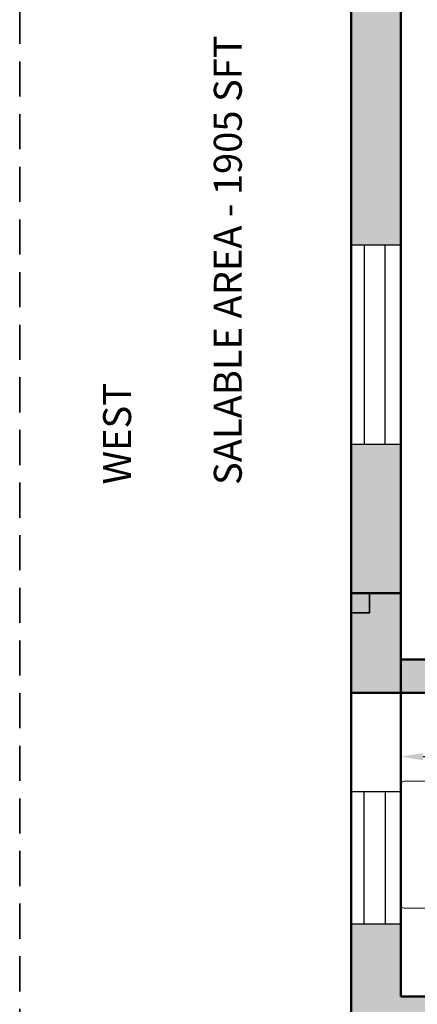
# Model space of a CAD drawing. Units: inches. Extents: x -7 to 1228, y -146 to 1091.
# Tile 50 of 88: x 0 to 72, y 786 to 964. Entities that reach past the tile are written whole.
import ezdxf

# ---------------------------------------------------------------- set-up
doc = ezdxf.new("R2010")
doc.units = ezdxf.units.IN
doc.linetypes.add('DASHED2', pattern=[9.525, 6.35, -3.175])
for name, color, linetype, lineweight in [('A-ANNO-DIMS', 2, 'Continuous', 18), ('A-ANNO-TEXT', 7, 'Continuous', 18), ('A-COLS', 6, 'Continuous', 35), ('A-FLOR-FIXT', 8, 'Continuous', 18), ('A-GLAZ', 175, 'Continuous', 25), ('A-WALL', 7, 'Continuous', 50), ('A-WALL-PATT', 251, 'Continuous', 13), ('C-PROP', 1, 'DASHED2', 35)]:
    doc.layers.add(name, color=color, linetype=linetype, lineweight=lineweight)
doc.styles.get("Standard").update_dxf_attribs({"font": 'arial.ttf'})
doc.dimstyles.new('ISO-25', dxfattribs={"dimtxt": 7, "dimasz": 4, "dimexe": 1.25, "dimexo": 0.625, "dimtad": 1, "dimdec": 1, "dimlunit": 3, "dimtxsty": 'Standard', "dimcen": 2.5, "dimadec": 0, "dimazin": 0, "dimtfac": 1, "dimtdec": 1, "dimtmove": 1, "dimatfit": 3, "dimfxl": 1, "dimarcsym": 0})

# ---------------------------------------------------------------- blocks, each defined once
blk = doc.blocks.new('A$C7B5C7CD4')
at = {"ltscale": 20}
for p, q in [((0, 0.614), (0, 0.4765)), ((0.243, 0.625), (0.011, 0.625)), ((0.243, 0.625), (0.475, 0.625)), ((0.486, 0.614), (0.486, 0.4765)), ((0.0212, 0.4467), (0.0946, 0.4214)), ((0.0946, 0.4214), (0.0576, 0.293)), ((0.0946, 0.4214), (0.1544, 0.4173)), ((0.3316, 0.4173), (0.1544, 0.4173)), ((0.3914, 0.4214), (0.3316, 0.4173)), ((0.4648, 0.4467), (0.3914, 0.4214)), ((0.3914, 0.4214), (0.4284, 0.293))]:
    blk.add_line(p, q, dxfattribs=at)
for centre, radius, start, end in [((0.011, 0.614), 0.011, 90, 180), ((0.475, 0.614), 0.011, 0, 90), ((0.0315, 0.4765), 0.0315, 180, 251), ((0.4545, 0.4765), 0.0315, 289, 0), ((0.24, 0.2602), 0.123, 88.6158, 131.7414), ((0.246, 0.2602), 0.123, 48.2586, 91.3842), ((0.2796, 0.219), 0.18, 132.4207, 213.289), ((0.2064, 0.219), 0.18, 326.711, 47.5793), ((0.2796, 0.219), 0.234, 161.5846, 212.8753), ((0.2064, 0.219), 0.234, 327.1247, 18.4154), ((0.243, 0.185), 0.131, 209.6292, 270), ((0.243, 0.185), 0.131, 270, 330.3708), ((0.243, 0.185), 0.185, 210.1745, 270), ((0.243, 0.185), 0.185, 270, 329.8255)]:
    blk.add_arc(centre, radius, start, end, dxfattribs=at)
for start, end in [(58.1785, 211.8215), (238.1785, 31.8215)]:
    blk.add_arc((0.2426, 0.2481), 0.0439, start, end)
blk = doc.blocks.new('WIN-36')
for p, q in [((0, 36), (0, 0)), ((9, 36), (0, 36)), ((2.34, 36), (2.34, 0)), ((6.14, 0), (6.14, 36)), ((9, 0), (9, 36)), ((0, 0), (9, 0)), ((2.34, 0), (6.14, 0))]:
    blk.add_line(p, q)
blk = doc.blocks.new('WIN-24')
for p, q in [((0, 0), (0, 24)), ((0, 24), (9, 24)), ((2.34, 0), (2.34, 24)), ((2.34, 24), (6.14, 24)), ((6.14, 24), (6.14, 0)), ((9, 24), (9, 0)), ((9, 0), (0, 0))]:
    blk.add_line(p, q)
blk = doc.blocks.new('*D28')
at = {"layer": 'A-ANNO-DIMS', "color": 0, "lineweight": -2, "transparency": 16777216}
for p, q in [((83.77, 830.42), (85.51, 836.22)), ((85.51, 836.22), (165.04, 836.22)), ((69, 826.61), (69, 831.67)), ((94.54, 830.42), (73, 830.42)), ((98.54, 826.61), (98.54, 831.67))]:
    blk.add_line(p, q, dxfattribs=at)
at = {"layer": 'A-ANNO-DIMS', "color": 0, "transparency": 16777216}
for points in [[(73, 831.08), (73, 829.75), (69, 830.42)], [(94.54, 831.08), (94.54, 829.75), (98.54, 830.42)]]:
    blk.add_solid(points, dxfattribs=at)
at = {"layer": 'Defpoints', "color": 0, "transparency": 16777216}
for p in [(69, 830.42), (69, 825.98), (98.54, 825.98)]:
    blk.add_point(p, dxfattribs=at)
at = {"layer": 'A-ANNO-DIMS', "color": 0, "transparency": 16777216, "insert": (125.27, 840.47), "char_height": 7, "attachment_point": 5}
blk.add_mtext('WC 2\'-5 1/2" TYP.', dxfattribs=at)

msp = doc.modelspace()

# ---------------------------------------------------------------- hatches: boundary and pattern name
at = {"layer": 'A-COLS'}
h = msp.add_hatch(color=256, dxfattribs=at)
h.dxf.hatch_style = 1
h.paths.add_polyline_path([(60, 842), (69, 842), (69, 860), (63.29, 860), (63.29, 856.45), (60, 856.45)])
h = msp.add_hatch(color=256, dxfattribs=at)
h.dxf.hatch_style = 1
h.paths.add_polyline_path([(63.29, 856.45), (63.29, 860), (60, 860), (60, 856.45)])
at = {"layer": 'A-WALL-PATT'}
h = msp.add_hatch(color=256, dxfattribs=at)
h.dxf.hatch_style = 1
h.paths.add_polyline_path([(69, 568), (60, 568), (60, 493), (63.29, 493), (69, 493)])
h.paths.add_polyline_path([(69, 662.41), (60, 662.41), (60, 586), (69, 586)], flags=17)
h.paths.add_polyline_path([(69, 723), (184, 723), (184, 734), (179, 734), (179, 728), (69, 728), (69, 741.62), (60, 741.62), (60, 698.41), (69, 698.41)], flags=17)
h.paths.add_polyline_path([(69, 782), (231, 782), (231, 728), (231, 723), (231, 586), (236, 586), (236, 787), (69, 787), (69, 800.13), (60, 800.13), (60, 765.62), (69, 765.62)])
h.paths.add_polyline_path([(184, 842), (189, 842), (189, 848), (173, 848), (173, 842), (179, 842), (179, 787), (184, 787)])
h.paths.add_polyline_path([(118.22, 69), (69, 69), (69, 60), (118.22, 60)])
h.paths.add_polyline_path([(227, 69), (154.22, 69), (154.22, 60), (227, 60)])
h.paths.add_polyline_path([(236, 60), (232.71, 60), (227, 60), (227, 36), (236, 36)])
h.paths.add_polyline_path([(389, 60), (380, 60), (380, 36), (389, 36)])
h.paths.add_polyline_path([(384, 181), (380, 181), (380, 115), (380, 78), (384, 78)])
h.paths.add_polyline_path([(380, 115), (334.55, 115), (334.55, 109), (380, 109)])
h.paths.add_polyline_path([(274.55, 115), (236, 115), (236, 201), (232.71, 201), (231, 201), (231, 78), (236, 78), (236, 109), (274.55, 109)])
h.paths.add_polyline_path([(69, 123), (60, 123), (60, 78), (69, 78)])
h.paths.add_polyline_path([(69, 201), (60, 201), (60, 159), (69, 159)])
h.paths.add_polyline_path([(143, 219), (69, 219), (69, 213), (143, 213)], flags=17)
h.paths.add_polyline_path([(189, 219), (184, 219), (184, 274), (231, 274), (231, 219), (236, 219), (236, 279), (184, 279), (184, 297), (179, 297), (179, 279), (69, 279), (69, 290.91), (60, 290.91), (60, 262.18), (69, 262.18), (69, 274), (179, 274), (179, 219), (173, 219), (173, 213), (189, 213)])
h.paths.add_polyline_path([(69, 238.18), (60, 238.18), (60, 219), (69, 219)], flags=17)
h.paths.add_polyline_path([(69, 333), (60, 333), (60, 314.91), (69, 314.91), (69, 316.96)])
h.paths.add_polyline_path([(190, 338), (184, 338), (69, 338), (69, 333), (179, 333), (179, 327), (184, 327), (184, 333.02), (190, 333.05)])
h.paths.add_polyline_path([(69, 386.81), (60, 386.81), (60, 351), (69, 351)])
h.paths.add_polyline_path([(69, 475), (60, 475), (60, 422.81), (69, 422.81)])
h.paths.add_polyline_path([(236, 475), (231, 475), (231, 351.24), (236, 351.24)])
h.paths.add_polyline_path([(384, 475), (380, 475), (380, 362), (384, 362)])
h.paths.add_polyline_path([(547, 307), (439, 307), (439, 356), (445, 356), (445, 362), (433, 362), (433, 307), (380, 307), (380, 244), (380, 241), (384, 241), (384, 301), (433, 301), (433, 277), (439, 277), (439, 301), (547, 301)])
h.paths.add_polyline_path([(547, 241), (439, 241), (439, 247), (433, 247), (433, 235), (547, 235)])
h.paths.add_polyline_path([(450, 69), (440.29, 69), (424.89, 69), (389, 69), (389, 60), (450, 60)])
h.paths.add_polyline_path([(547, 69), (486, 69), (486, 60), (547, 60)])
h.paths.add_polyline_path([(556, 148.27), (547, 148.27), (547, 78), (556, 78)])
h.paths.add_polyline_path([(556, 223), (547, 223), (547, 195), (547, 184.27), (556, 184.27)])
h.paths.add_polyline_path([(556, 311.19), (547, 311.19), (547, 273.08), (556, 273.08)])
h.paths.add_polyline_path([(556, 344), (552.71, 344), (547, 344), (547, 335.19), (556, 335.19)])
h.paths.add_polyline_path([(556, 249.08), (547, 249.08), (547, 241), (556, 241)])
h.paths.add_polyline_path([(547, 362), (475, 362), (475, 356), (547, 356)], flags=0)
h.paths.add_polyline_path([(556, 399.62), (547, 399.62), (547, 362), (556, 362)])
h.paths.add_polyline_path([(556, 475), (547, 475), (547, 435.62), (556, 435.62)])
h.paths.add_polyline_path([(547, 493), (389, 493), (389, 487), (547, 487)])
h.paths.add_polyline_path([(380, 493), (278, 493), (278, 487), (380, 487)])
h.paths.add_polyline_path([(227, 493), (69, 493), (69, 487), (227, 487)])
h.paths.add_polyline_path([(643, 122.44), (634, 122.44), (634, 78), (643, 78)])
h.paths.add_polyline_path([(702.5, 69), (692.79, 69), (677.39, 69), (643, 69), (643, 60), (702.5, 60)])
h.paths.add_polyline_path([(798, 69), (738.5, 69), (738.5, 60), (798, 60)])
h.paths.add_polyline_path([(807, 60), (803.71, 60), (798, 60), (798, 36), (807, 36)])
h.paths.add_polyline_path([(807, 109), (846.75, 109), (846.75, 115), (807, 115), (807, 159), (802, 159), (802, 78), (807, 78)])
h.paths.add_polyline_path([(807, 201), (802, 201), (802, 195), (807, 195)])
h.paths.add_polyline_path([(643, 201), (634, 201), (634, 158.44), (643, 158.44)])
h.paths.add_polyline_path([(756, 225), (751, 225), (751, 219), (643, 219), (643, 213), (756, 213)])
h.paths.add_polyline_path([(643, 240.85), (634, 240.85), (634, 219), (643, 219)])
h.paths.add_polyline_path([(643, 274), (643, 288.63), (634, 288.63), (634, 264.85), (643, 264.85)])
h.paths.add_polyline_path([(802, 279), (756, 279), (756, 297), (751, 297), (751, 279), (643, 279), (643, 274), (751, 274), (751, 255), (756, 255), (756, 274), (802, 274)])
h.paths.add_polyline_path([(807, 333), (803.71, 333), (802, 333), (802, 279), (802, 274), (802, 219), (807, 219)])
h.paths.add_polyline_path([(956, 182), (951, 182), (951, 115), (906.75, 115), (906.75, 109), (951, 109), (951, 78), (956, 78)])
h.paths.add_polyline_path([(960, 60), (951, 60), (951, 36), (960, 36)])
h.paths.add_polyline_path([(1021, 69), (1005.78, 69), (960, 69), (960, 60), (1021, 60)])
h.paths.add_polyline_path([(956, 224), (951, 224), (951, 218), (956, 218)])
h.paths.add_polyline_path([(956, 302), (1004, 302), (1004, 278), (1010, 278), (1010, 302), (1118, 302), (1118, 290.81), (1127, 290.81), (1127, 326.97), (1118, 326.97), (1118, 320.97), (1118, 307), (1010, 307), (1010, 356), (1016, 356), (1016, 362), (1004, 362), (1004, 307), (951, 307), (951, 244), (951, 242), (954.29, 242), (956, 242)])
h.paths.add_polyline_path([(643, 333), (634, 333), (634, 312.63), (643, 312.63), (643, 316.96)])
h.paths.add_polyline_path([(756, 338), (643, 338), (643, 333), (751, 333), (751, 327), (756, 327)])
h.paths.add_polyline_path([(643, 388), (634, 388), (634, 351), (643, 351)])
h.paths.add_polyline_path([(807, 357), (802, 357), (802, 351), (807, 351)])
h.paths.add_polyline_path([(807, 475), (802, 475), (802, 393), (807, 393)])
h.paths.add_polyline_path([(643, 475), (634, 475), (634, 424), (643, 424)])
h.paths.add_polyline_path([(798, 493), (643, 493), (643, 487), (798, 487)])
h.paths.add_polyline_path([(634, 493), (556, 493), (556, 487), (634, 487)])
h.paths.add_polyline_path([(813, 493), (807, 493), (807, 487), (813, 487)])
h.paths.add_polyline_path([(951, 493), (849, 493), (849, 487), (951, 487)])
h.paths.add_polyline_path([(956, 484), (951, 484), (951, 374), (956, 374)])
h.paths.add_polyline_path([(1109, 493), (969, 493), (969, 487), (1109, 487)])
h.paths.add_polyline_path([(1127, 484), (1118, 484), (1118, 450.64), (1127, 450.64)])
h.paths.add_polyline_path([(1127, 414.64), (1118, 414.64), (1118, 365), (1127, 365)])
h.paths.add_polyline_path([(1109, 362), (1046, 362), (1046, 356), (1109, 356)], flags=17)
h.paths.add_polyline_path([(1127, 356), (1123.45, 356), (1118, 356), (1118, 350.97), (1127, 350.97)], flags=0)
h.paths.add_polyline_path([(1127, 266.81), (1118, 266.81), (1118, 262.36), (1118, 242), (1127, 242)], flags=17)
h.paths.add_polyline_path([(1118, 242), (1010, 242), (1010, 248), (1004, 248), (1004, 237), (1118, 237)])
h.paths.add_polyline_path([(1127, 224), (1118, 224), (1118, 170), (1127, 170)])
h.paths.add_polyline_path([(1127, 134), (1118, 134), (1118, 78), (1127, 78)])
h.paths.add_polyline_path([(1118, 69), (1057, 69), (1057, 60), (1118, 60)])
h.paths.add_polyline_path([(227, 571.55), (227, 574), (69, 574), (69, 568), (227, 568)])
h.paths.add_polyline_path([(380, 571.55), (380, 574), (278, 574), (278, 568), (380, 568)])
h.paths.add_polyline_path([(242, 574), (236, 574), (236, 568), (242, 568)])
h.paths.add_polyline_path([(547, 571.55), (547, 574), (389, 574), (389, 568), (547, 568)])
h.paths.add_polyline_path([(384, 733), (380, 733), (380, 586), (384, 586)])
h.paths.add_polyline_path([(556, 646), (634, 646), (634, 655), (547, 655), (547, 586), (556, 586)])
h.paths.add_polyline_path([(634, 574), (556, 574), (556, 568), (634, 568)])
h.paths.add_polyline_path([(643, 655), (634, 655), (634, 586), (643, 586)])
h.paths.add_polyline_path([(798, 574), (643, 574), (643, 568), (798, 568)])
h.paths.add_polyline_path([(643, 663.85), (634, 663.85), (634, 655), (643, 655)])
h.paths.add_polyline_path([(556, 676.97), (547, 676.97), (547, 655), (556, 655)])
h.paths.add_polyline_path([(556, 733), (547, 733), (547, 712.97), (556, 712.97)])
h.paths.add_polyline_path([(643, 710), (634, 710), (634, 699.85), (643, 699.85)])
h.paths.add_polyline_path([(807, 668), (802, 668), (802, 586), (807, 586)])
h.paths.add_polyline_path([(951, 574), (849, 574), (849, 568), (951, 568)])
h.paths.add_polyline_path([(956, 691), (951, 691), (951, 577), (956, 577)])
h.paths.add_polyline_path([(1109, 574), (969, 574), (969, 568), (1109, 568)])
h.paths.add_polyline_path([(1127, 643.4), (1118, 643.4), (1118, 577), (1127, 577)])
h.paths.add_polyline_path([(1127, 568), (1123.45, 568), (1118, 568), (1118, 493), (1127, 493)])
h.paths.add_polyline_path([(1127, 733), (1118, 733), (1118, 679.4), (1127, 679.4)])
h.paths.add_polyline_path([(1127, 777.35), (1118, 777.35), (1118, 770.04), (1118, 751), (1127, 751)], flags=17)
h.paths.add_polyline_path([(1118, 751), (1010, 751), (1010, 757), (1004, 757), (1004, 745), (1118, 745)])
h.paths.add_polyline_path([(956, 811), (1004, 811), (1004, 787), (1010, 787), (1010, 811), (1017.87, 811), (1017.87, 811.63, -0.414214), (1018.25, 812), (1031.98, 812, -0.414214), (1032.35, 811.63), (1032.35, 811), (1118, 811), (1118, 801.35), (1127, 801.35), (1127, 834.69), (1118, 834.69), (1118, 830.24), (1118, 817), (1010, 817), (1010, 866), (1016, 866), (1016, 872), (1004, 872), (1004, 817), (956, 817), (956, 866), (951, 866), (951, 751), (954.29, 751), (956, 751)])
h.paths.add_polyline_path([(1118, 872), (1046, 872), (1046, 866), (1118, 866)], flags=17)
h.paths.add_polyline_path([(1127, 924.71), (1118, 924.71), (1118, 884), (1127, 884)])
h.paths.add_polyline_path([(1127, 866), (1123.71, 866), (1118, 866), (1118, 858.69), (1127, 858.69)], flags=17)
h.paths.add_polyline_path([(956, 983), (951, 983), (951, 952), (807, 952), (807, 983), (802, 983), (802, 902), (807, 902), (807, 946), (951, 946), (951, 884), (956, 884)])
h.paths.add_polyline_path([(807, 842), (802, 842), (802, 787), (756, 787), (756, 806), (751, 806), (751, 787), (643, 787), (643, 782), (751, 782), (751, 764), (756, 764), (756, 782), (802, 782), (802, 728), (807, 728)])
h.paths.add_polyline_path([(756, 848), (643, 848), (643, 842), (751, 842), (751, 836), (756, 836)])
h.paths.add_polyline_path([(756, 734), (751, 734), (751, 728), (643, 728), (643, 723), (756, 723)])
h.paths.add_polyline_path([(643, 749.79), (634, 749.79), (634, 728), (637.29, 728), (643, 728)])
h.paths.add_polyline_path([(643, 805.41), (634, 805.41), (634, 773.79), (643, 773.79)])
h.paths.add_polyline_path([(643, 896.66), (634, 896.66), (634, 860), (637.29, 860), (643, 860)])
h.paths.add_polyline_path([(643, 842), (634, 842), (634, 829.41), (643, 829.41)])
h.paths.add_polyline_path([(643, 983), (634, 983), (634, 932.66), (643, 932.66)])
h.paths.add_polyline_path([(1127, 983), (1118, 983), (1118, 960.71), (1127, 960.71)])
h.paths.add_polyline_path([(1118, 1001), (1077.53, 1001), (1077.53, 992), (1118, 992)])
h.paths.add_polyline_path([(1041.53, 1001), (960, 1001), (960, 992), (1041.53, 992)])
h.paths.add_polyline_path([(960, 1025), (951, 1025), (951, 1001), (954.29, 1001), (960, 1001)])
h.paths.add_polyline_path([(807, 1025), (798, 1025), (798, 1001), (807, 1001)])
h.paths.add_polyline_path([(798, 1001), (738.5, 1001), (738.5, 992), (798, 992)])
h.paths.add_polyline_path([(702.5, 1001), (643, 1001), (643, 992), (702.5, 992)])
h.paths.add_polyline_path([(547, 1001), (499.11, 1001), (499.11, 992), (547, 992)])
h.paths.add_polyline_path([(463.11, 1001), (389, 1001), (389, 992), (463.11, 992)])
h.paths.add_polyline_path([(389, 1025), (380, 1025), (380, 1022), (380, 1001), (383.29, 1001), (389, 1001)])
h.paths.add_polyline_path([(236, 1025), (227, 1025), (227, 1001), (236, 1001)])
h.paths.add_polyline_path([(236, 983), (231, 983), (231, 860), (236, 860)])
h.paths.add_polyline_path([(274.55, 952), (236, 952), (236, 946), (274.55, 946)])
h.paths.add_polyline_path([(380, 952), (334.55, 952), (334.55, 946), (380, 946)])
h.paths.add_polyline_path([(384, 983), (380, 983), (380, 884), (383.29, 884), (384, 884)])
h.paths.add_polyline_path([(227, 1001), (155.01, 1001), (155.01, 992), (162.87, 992), (227, 992)])
h.paths.add_polyline_path([(119.01, 1001), (69, 1001), (69, 992), (119.01, 992)])
h.paths.add_polyline_path([(69, 983), (60, 983), (60, 922.99), (69, 922.99)])
h.paths.add_polyline_path([(69, 886.99), (60, 886.99), (60, 860), (63.29, 860), (69, 860)])
h.paths.add_polyline_path([(143, 848), (69, 848), (69, 842), (143, 842)])

# ---------------------------------------------------------------- linework, layer by layer
at = {"layer": 'A-COLS'}
msp.add_lwpolyline([(60, 860), (63.29, 860), (63.29, 856.45), (60, 856.45)], close=True, dxfattribs=at)
at = {"layer": 'A-WALL'}
for p, q in [((60, 1001), (60, 60)), ((69, 992), (69, 848)), ((60, 860), (69, 860)), ((60, 842), (60, 860)), ((69, 860), (69, 842)), ((143, 848), (69, 848)), ((69, 842), (60, 842)), ((69, 842), (69, 787)), ((143, 842), (69, 842)), ((236, 787), (69, 787))]:
    msp.add_line(p, q, dxfattribs=at)
at = {"layer": 'C-PROP'}
msp.add_line((0, 1061), (0, 0), dxfattribs=at)

# ---------------------------------------------------------------- block references
at = {"layer": 'A-FLOR-FIXT', "xscale": 47.26153857112405, "yscale": 47.26153857112405, "zscale": 47.26153857112405, "rotation": 90}
msp.add_blockref('A$C7B5C7CD4', (98.54, 803.02), dxfattribs=at)
at = {"layer": 'A-GLAZ'}
for name, p in [('WIN-36', (60, 886.99)), ('WIN-24', (60, 800.13))]:
    msp.add_blockref(name, p, dxfattribs=at)

# ---------------------------------------------------------------- texts
at = {"layer": 'A-ANNO-TEXT', "attachment_point": 1, "rotation": 90}
for s, insert, char_height in [('{SALABLE AREA - 1905 SFT}', (35.13, 879.59), 5.0568), ('WEST', (15.1, 879.69), 5.057)]:
    msp.add_mtext_dynamic_manual_height_columns(s, width=137.2821, gutter_width=25.28, heights=[0], dxfattribs=dict(at, insert=insert, char_height=char_height))

# ---------------------------------------------------------------- dimensions: what is measured, and where the dimension line sits
at = {"layer": 'A-ANNO-DIMS'}
dim = msp.add_linear_dim(base=(69, 830.42), p1=(98.54, 825.98), p2=(69, 825.98), angle=180, text='WC <> TYP.', dimstyle='ISO-25', override={"dimdec": 1, "dimlfac": 1, "dimrnd": 0, "dimzin": 1, "dimdsep": 46, "dimlunit": 4, "dimfrac": 2}, dxfattribs=at)
dim.commit()
dim.dimension.update_dxf_attribs({"geometry": '*D28', "text_midpoint": (86.14, 840.47)})

doc.saveas('drawing.dxf')
